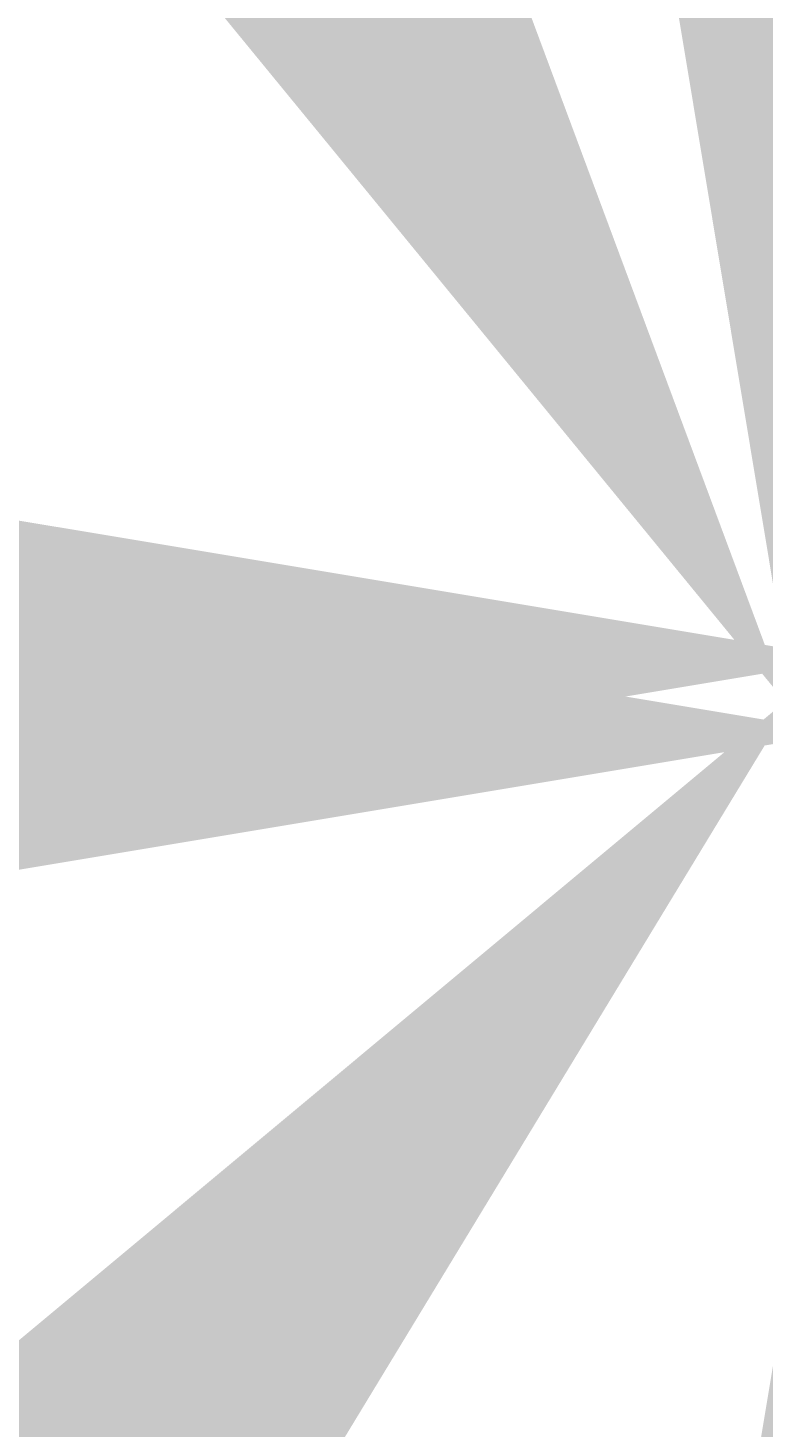
# Model space of a CAD drawing. Units: millimetres. Extents: x -22994 to 29398, y -19990 to 20176.
# Tile 4 of 135: x -2139 to -44, y -1986 to 2002. Entities that reach past the tile are written whole.
import ezdxf

# ---------------------------------------------------------------- set-up
doc = ezdxf.new("R2010")
doc.units = ezdxf.units.MM
doc.header["$MEASUREMENT"] = 0
doc.layers.add('M-DIMS', color=2, linetype='Continuous', lineweight=18)
doc.styles.get("Standard").update_dxf_attribs({"font": 'arial.ttf'})
doc.dimstyles.get("Standard").update_dxf_attribs({"dimtxt": 0.18, "dimasz": 10000, "dimexe": 0.18, "dimexo": 0.0625, "dimgap": 0.09, "dimtad": 0, "dimtih": 1, "dimtoh": 1, "dimdec": 0, "dimzin": 0, "dimdsep": 46, "dimtxsty": 'Standard', "dimcen": 0.09, "dimadec": 0, "dimazin": 0, "dimtfac": 1, "dimtdec": 0, "dimtofl": 0, "dimtmove": 0, "dimatfit": 3, "dimfxl": 1, "dimtolj": 1, "dimtzin": 0, "dimlwd": 30, "dimarcsym": 0})

# ---------------------------------------------------------------- blocks, each defined once
blk = doc.blocks.new('*D2')
at = {"layer": 'Defpoints', "color": 0, "transparency": 16777216}
for p in [(6.7, 10.3), (290.9, 10.3), (290.9, -5.1)]:
    blk.add_point(p, dxfattribs=at)
at = {"layer": 'M-DIMS', "color": 0, "lineweight": -2, "transparency": 16777216}
for p, q in [((6.7, 10.2), (6.7, -5.3)), ((290.9, 10.2), (290.9, -5.3))]:
    blk.add_line(p, q, dxfattribs=at)
at = {"layer": 'M-DIMS', "color": 0, "lineweight": 30, "transparency": 16777216}
for p, q in [((-9993.3, -5.1), (-19993.3, -5.1)), ((10290.9, -5.1), (20290.9, -5.1))]:
    blk.add_line(p, q, dxfattribs=at)
at = {"layer": 'M-DIMS', "color": 0, "transparency": 16777216}
for points in [[(-9993.3, 1661.6), (-9993.3, -1671.7), (6.7, -5.1)], [(10290.9, 1661.6), (10290.9, -1671.7), (290.9, -5.1)]]:
    blk.add_solid(points, dxfattribs=at)
at = {"layer": 'M-DIMS', "color": 0, "transparency": 16777216, "insert": (148.8, -5.1), "char_height": 0.18, "attachment_point": 5}
blk.add_mtext('\\A1;284.2', dxfattribs=at)
blk = doc.blocks.new('*D3')
at = {"layer": 'Defpoints', "color": 0, "transparency": 16777216}
for p in [(110.3, 204.2), (110.3, 176.4), (95.8, 128)]:
    blk.add_point(p, dxfattribs=at)
at = {"layer": 'M-DIMS', "color": 0, "lineweight": 30, "transparency": 16777216}
for p, q in [((-9904.2, 204.2), (-19904.2, 204.2)), ((10110.3, 204.2), (20110.3, 204.2))]:
    blk.add_line(p, q, dxfattribs=at)
at = {"layer": 'M-DIMS', "color": 0, "lineweight": -2, "transparency": 16777216}
for p, q in [((95.8, 128), (95.8, 204.3)), ((110.3, 176.4), (110.3, 204.3))]:
    blk.add_line(p, q, dxfattribs=at)
at = {"layer": 'M-DIMS', "color": 0, "transparency": 16777216}
for points in [[(-9904.2, 1870.8), (-9904.2, -1462.5), (95.8, 204.2)], [(10110.3, 1870.8), (10110.3, -1462.5), (110.3, 204.2)]]:
    blk.add_solid(points, dxfattribs=at)
at = {"layer": 'M-DIMS', "color": 0, "transparency": 16777216, "insert": (103, 204.2), "char_height": 0.18, "attachment_point": 5}
blk.add_mtext('\\A1;14.432', dxfattribs=at)
blk = doc.blocks.new('*D4')
at = {"layer": 'Defpoints', "color": 0, "transparency": 16777216}
for p in [(116.3, 204.2), (110.3, 176.4), (116.3, 176.4)]:
    blk.add_point(p, dxfattribs=at)
at = {"layer": 'M-DIMS', "color": 0, "lineweight": 30, "transparency": 16777216}
for p, q in [((-9889.7, 204.2), (-19889.7, 204.2)), ((10116.3, 204.2), (20116.3, 204.2))]:
    blk.add_line(p, q, dxfattribs=at)
at = {"layer": 'M-DIMS', "color": 0, "lineweight": -2, "transparency": 16777216}
for p, q in [((110.3, 176.4), (110.3, 204.3)), ((116.3, 176.4), (116.3, 204.3))]:
    blk.add_line(p, q, dxfattribs=at)
at = {"layer": 'M-DIMS', "color": 0, "transparency": 16777216}
for points in [[(-9889.7, 1870.8), (-9889.7, -1462.5), (110.3, 204.2)], [(10116.3, 1870.8), (10116.3, -1462.5), (116.3, 204.2)]]:
    blk.add_solid(points, dxfattribs=at)
at = {"layer": 'M-DIMS', "color": 0, "transparency": 16777216, "insert": (113.3, 204.2), "char_height": 0.18, "attachment_point": 5}
blk.add_mtext('\\A1;6', dxfattribs=at)
blk = doc.blocks.new('*D5')
at = {"layer": 'Defpoints', "color": 0, "transparency": 16777216}
for p in [(181.3, 204.2), (116.3, 176.4), (181.3, 176.4)]:
    blk.add_point(p, dxfattribs=at)
at = {"layer": 'M-DIMS', "color": 0, "lineweight": 30, "transparency": 16777216}
for p, q in [((-9883.7, 204.2), (-19883.7, 204.2)), ((10181.3, 204.2), (20181.3, 204.2))]:
    blk.add_line(p, q, dxfattribs=at)
at = {"layer": 'M-DIMS', "color": 0, "lineweight": -2, "transparency": 16777216}
for p, q in [((116.3, 176.4), (116.3, 204.3)), ((181.3, 176.4), (181.3, 204.3))]:
    blk.add_line(p, q, dxfattribs=at)
at = {"layer": 'M-DIMS', "color": 0, "transparency": 16777216}
for points in [[(-9883.7, 1870.8), (-9883.7, -1462.5), (116.3, 204.2)], [(10181.3, 1870.8), (10181.3, -1462.5), (181.3, 204.2)]]:
    blk.add_solid(points, dxfattribs=at)
at = {"layer": 'M-DIMS', "color": 0, "transparency": 16777216, "insert": (148.8, 204.2), "char_height": 0.18, "attachment_point": 5}
blk.add_mtext('\\A1;65', dxfattribs=at)
blk = doc.blocks.new('*D6')
at = {"layer": 'Defpoints', "color": 0, "transparency": 16777216}
for p in [(187.3, 204.2), (181.3, 176.4), (187.3, 176.4)]:
    blk.add_point(p, dxfattribs=at)
at = {"layer": 'M-DIMS', "color": 0, "lineweight": 30, "transparency": 16777216}
for p, q in [((-9818.7, 204.2), (-19818.7, 204.2)), ((10187.3, 204.2), (20187.3, 204.2))]:
    blk.add_line(p, q, dxfattribs=at)
at = {"layer": 'M-DIMS', "color": 0, "lineweight": -2, "transparency": 16777216}
for p, q in [((181.3, 176.4), (181.3, 204.3)), ((187.3, 176.4), (187.3, 204.3))]:
    blk.add_line(p, q, dxfattribs=at)
at = {"layer": 'M-DIMS', "color": 0, "transparency": 16777216}
for points in [[(-9818.7, 1870.8), (-9818.7, -1462.5), (181.3, 204.2)], [(10187.3, 1870.8), (10187.3, -1462.5), (187.3, 204.2)]]:
    blk.add_solid(points, dxfattribs=at)
at = {"layer": 'M-DIMS', "color": 0, "transparency": 16777216, "insert": (184.3, 204.2), "char_height": 0.18, "attachment_point": 5}
blk.add_mtext('\\A1;6', dxfattribs=at)
blk = doc.blocks.new('*D7')
at = {"layer": 'Defpoints', "color": 0, "transparency": 16777216}
for p in [(201.7, 204.2), (187.3, 176.4), (201.7, 128)]:
    blk.add_point(p, dxfattribs=at)
at = {"layer": 'M-DIMS', "color": 0, "lineweight": 30, "transparency": 16777216}
for p, q in [((-9812.7, 204.2), (-19812.7, 204.2)), ((10201.7, 204.2), (20201.7, 204.2))]:
    blk.add_line(p, q, dxfattribs=at)
at = {"layer": 'M-DIMS', "color": 0, "lineweight": -2, "transparency": 16777216}
for p, q in [((187.3, 176.4), (187.3, 204.3)), ((201.7, 128), (201.7, 204.3))]:
    blk.add_line(p, q, dxfattribs=at)
at = {"layer": 'M-DIMS', "color": 0, "transparency": 16777216}
for points in [[(-9812.7, 1870.8), (-9812.7, -1462.5), (187.3, 204.2)], [(10201.7, 1870.8), (10201.7, -1462.5), (201.7, 204.2)]]:
    blk.add_solid(points, dxfattribs=at)
at = {"layer": 'M-DIMS', "color": 0, "transparency": 16777216, "insert": (194.5, 204.2), "char_height": 0.18, "attachment_point": 5}
blk.add_mtext('\\A1;14.432', dxfattribs=at)
blk = doc.blocks.new('*D8')
at = {"layer": 'Defpoints', "color": 0, "transparency": 16777216}
for p in [(227.6, 204.2), (201.7, 128), (227.6, 146.7)]:
    blk.add_point(p, dxfattribs=at)
at = {"layer": 'M-DIMS', "color": 0, "lineweight": 30, "transparency": 16777216}
for p, q in [((-9798.3, 204.2), (-19798.3, 204.2)), ((10227.6, 204.2), (20227.6, 204.2))]:
    blk.add_line(p, q, dxfattribs=at)
at = {"layer": 'M-DIMS', "color": 0, "lineweight": -2, "transparency": 16777216}
for p, q in [((201.7, 128), (201.7, 204.3)), ((227.6, 146.8), (227.6, 204.3))]:
    blk.add_line(p, q, dxfattribs=at)
at = {"layer": 'M-DIMS', "color": 0, "transparency": 16777216}
for points in [[(-9798.3, 1870.8), (-9798.3, -1462.5), (201.7, 204.2)], [(10227.6, 1870.8), (10227.6, -1462.5), (227.6, 204.2)]]:
    blk.add_solid(points, dxfattribs=at)
at = {"layer": 'M-DIMS', "color": 0, "transparency": 16777216, "insert": (214.7, 204.2), "char_height": 0.18, "attachment_point": 5}
blk.add_mtext('\\A1;25.95', dxfattribs=at)
blk = doc.blocks.new('*D9')
at = {"layer": 'Defpoints', "color": 0, "transparency": 16777216}
for p in [(187.3, 176.4), (306.2, 176.4), (290.9, 10.3)]:
    blk.add_point(p, dxfattribs=at)
at = {"layer": 'M-DIMS', "color": 0, "lineweight": 30, "transparency": 16777216}
for p, q in [((306.2, 10176.4), (306.2, 20176.4)), ((306.2, -9989.7), (306.2, -19989.7))]:
    blk.add_line(p, q, dxfattribs=at)
at = {"layer": 'M-DIMS', "color": 0, "lineweight": -2, "transparency": 16777216}
for p, q in [((187.3, 176.4), (306.4, 176.4)), ((290.9, 10.3), (306.4, 10.3))]:
    blk.add_line(p, q, dxfattribs=at)
at = {"layer": 'M-DIMS', "color": 0, "transparency": 16777216}
for points in [[(-1360.5, 10176.4), (1972.9, 10176.4), (306.2, 176.4)], [(-1360.5, -9989.7), (1972.9, -9989.7), (306.2, 10.3)]]:
    blk.add_solid(points, dxfattribs=at)
at = {"layer": 'M-DIMS', "color": 0, "transparency": 16777216, "insert": (306.2, 93.3), "char_height": 0.18, "attachment_point": 5}
blk.add_mtext('\\A1;166.1', dxfattribs=at)
blk = doc.blocks.new('*D10')
at = {"layer": 'Defpoints', "color": 0, "transparency": 16777216}
for p in [(125.6, 136.1), (133.3, 136.1), (133.3, -5.1)]:
    blk.add_point(p, dxfattribs=at)
at = {"layer": 'M-DIMS', "color": 0, "lineweight": -2, "transparency": 16777216}
for p, q in [((125.6, 136), (125.6, -5.3)), ((133.3, 136), (133.3, -5.3))]:
    blk.add_line(p, q, dxfattribs=at)
at = {"layer": 'M-DIMS', "color": 0, "lineweight": 30, "transparency": 16777216}
for p, q in [((-9874.4, -5.1), (-19874.4, -5.1)), ((10133.3, -5.1), (20133.3, -5.1))]:
    blk.add_line(p, q, dxfattribs=at)
at = {"layer": 'M-DIMS', "color": 0, "transparency": 16777216}
for points in [[(-9874.4, 1661.6), (-9874.4, -1671.7), (125.6, -5.1)], [(10133.3, 1661.6), (10133.3, -1671.7), (133.3, -5.1)]]:
    blk.add_solid(points, dxfattribs=at)
at = {"layer": 'M-DIMS', "color": 0, "transparency": 16777216, "insert": (129.5, -5.1), "char_height": 0.18, "attachment_point": 5}
blk.add_mtext('\\A1;7.696', dxfattribs=at)
blk = doc.blocks.new('*D11')
at = {"layer": 'Defpoints', "color": 0, "transparency": 16777216}
for p in [(133.3, 136.1), (135.6, 136.1), (135.6, -5.1)]:
    blk.add_point(p, dxfattribs=at)
at = {"layer": 'M-DIMS', "color": 0, "lineweight": -2, "transparency": 16777216}
for p, q in [((133.3, 136), (133.3, -5.3)), ((135.6, 136), (135.6, -5.3))]:
    blk.add_line(p, q, dxfattribs=at)
at = {"layer": 'M-DIMS', "color": 0, "lineweight": 30, "transparency": 16777216}
for p, q in [((-9866.7, -5.1), (-19866.7, -5.1)), ((10135.6, -5.1), (20135.6, -5.1))]:
    blk.add_line(p, q, dxfattribs=at)
at = {"layer": 'M-DIMS', "color": 0, "transparency": 16777216}
for points in [[(-9866.7, 1661.6), (-9866.7, -1671.7), (133.3, -5.1)], [(10135.6, 1661.6), (10135.6, -1671.7), (135.6, -5.1)]]:
    blk.add_solid(points, dxfattribs=at)
at = {"layer": 'M-DIMS', "color": 0, "transparency": 16777216, "insert": (134.5, -5.1), "char_height": 0.18, "attachment_point": 5}
blk.add_mtext('\\A1;2.304', dxfattribs=at)
blk = doc.blocks.new('*D12')
at = {"layer": 'Defpoints', "color": 0, "transparency": 16777216}
for p in [(135.6, 136.1), (145.6, 136.1), (145.6, -5.1)]:
    blk.add_point(p, dxfattribs=at)
at = {"layer": 'M-DIMS', "color": 0, "lineweight": -2, "transparency": 16777216}
for p, q in [((135.6, 136), (135.6, -5.3)), ((145.6, 136), (145.6, -5.3))]:
    blk.add_line(p, q, dxfattribs=at)
at = {"layer": 'M-DIMS', "color": 0, "lineweight": 30, "transparency": 16777216}
for p, q in [((-9864.4, -5.1), (-19864.4, -5.1)), ((10145.6, -5.1), (20145.6, -5.1))]:
    blk.add_line(p, q, dxfattribs=at)
at = {"layer": 'M-DIMS', "color": 0, "transparency": 16777216}
for points in [[(-9864.4, 1661.6), (-9864.4, -1671.7), (135.6, -5.1)], [(10145.6, 1661.6), (10145.6, -1671.7), (145.6, -5.1)]]:
    blk.add_solid(points, dxfattribs=at)
at = {"layer": 'M-DIMS', "color": 0, "transparency": 16777216, "insert": (140.6, -5.1), "char_height": 0.18, "attachment_point": 5}
blk.add_mtext('\\A1;10', dxfattribs=at)
blk = doc.blocks.new('*D13')
at = {"layer": 'Defpoints', "color": 0, "transparency": 16777216}
for p in [(145.6, 136.1), (155.6, 136.1), (155.6, -5.1)]:
    blk.add_point(p, dxfattribs=at)
at = {"layer": 'M-DIMS', "color": 0, "lineweight": -2, "transparency": 16777216}
for p, q in [((145.6, 136), (145.6, -5.3)), ((155.6, 136), (155.6, -5.3))]:
    blk.add_line(p, q, dxfattribs=at)
at = {"layer": 'M-DIMS', "color": 0, "lineweight": 30, "transparency": 16777216}
for p, q in [((-9854.4, -5.1), (-19854.4, -5.1)), ((10155.6, -5.1), (20155.6, -5.1))]:
    blk.add_line(p, q, dxfattribs=at)
at = {"layer": 'M-DIMS', "color": 0, "transparency": 16777216}
for points in [[(-9854.4, 1661.6), (-9854.4, -1671.7), (145.6, -5.1)], [(10155.6, 1661.6), (10155.6, -1671.7), (155.6, -5.1)]]:
    blk.add_solid(points, dxfattribs=at)
at = {"layer": 'M-DIMS', "color": 0, "transparency": 16777216, "insert": (150.6, -5.1), "char_height": 0.18, "attachment_point": 5}
blk.add_mtext('\\A1;10', dxfattribs=at)
blk = doc.blocks.new('*D14')
at = {"layer": 'Defpoints', "color": 0, "transparency": 16777216}
for p in [(155.6, 136.1), (165.6, 136.1), (165.6, -5.1)]:
    blk.add_point(p, dxfattribs=at)
at = {"layer": 'M-DIMS', "color": 0, "lineweight": -2, "transparency": 16777216}
for p, q in [((155.6, 136), (155.6, -5.3)), ((165.6, 136), (165.6, -5.3))]:
    blk.add_line(p, q, dxfattribs=at)
at = {"layer": 'M-DIMS', "color": 0, "lineweight": 30, "transparency": 16777216}
for p, q in [((-9844.4, -5.1), (-19844.4, -5.1)), ((10165.6, -5.1), (20165.6, -5.1))]:
    blk.add_line(p, q, dxfattribs=at)
at = {"layer": 'M-DIMS', "color": 0, "transparency": 16777216}
for points in [[(-9844.4, 1661.6), (-9844.4, -1671.7), (155.6, -5.1)], [(10165.6, 1661.6), (10165.6, -1671.7), (165.6, -5.1)]]:
    blk.add_solid(points, dxfattribs=at)
at = {"layer": 'M-DIMS', "color": 0, "transparency": 16777216, "insert": (160.6, -5.1), "char_height": 0.18, "attachment_point": 5}
blk.add_mtext('\\A1;10', dxfattribs=at)
blk = doc.blocks.new('*D15')
at = {"layer": 'Defpoints', "color": 0, "transparency": 16777216}
for p in [(173.3, 154.8), (173.3, 136.1), (306.2, 136.1)]:
    blk.add_point(p, dxfattribs=at)
at = {"layer": 'M-DIMS', "color": 0, "lineweight": 30, "transparency": 16777216}
for p, q in [((306.2, 10154.8), (306.2, 20154.8)), ((306.2, -9863.9), (306.2, -19863.9))]:
    blk.add_line(p, q, dxfattribs=at)
at = {"layer": 'M-DIMS', "color": 0, "lineweight": -2, "transparency": 16777216}
for p, q in [((173.4, 154.8), (306.4, 154.8)), ((173.4, 136.1), (306.4, 136.1))]:
    blk.add_line(p, q, dxfattribs=at)
at = {"layer": 'M-DIMS', "color": 0, "transparency": 16777216}
for points in [[(-1360.5, 10154.8), (1972.9, 10154.8), (306.2, 154.8)], [(-1360.5, -9863.9), (1972.9, -9863.9), (306.2, 136.1)]]:
    blk.add_solid(points, dxfattribs=at)
at = {"layer": 'M-DIMS', "color": 0, "transparency": 16777216, "insert": (306.2, 145.4), "char_height": 0.18, "attachment_point": 5}
blk.add_mtext('\\A1;18.717', dxfattribs=at)
blk = doc.blocks.new('*D16')
at = {"layer": 'Defpoints', "color": 0, "transparency": 16777216}
for p in [(120.2, 204.2), (110.5, 48), (120.2, 48)]:
    blk.add_point(p, dxfattribs=at)
at = {"layer": 'M-DIMS', "color": 0, "lineweight": 30, "transparency": 16777216}
for p, q in [((-9889.5, 204.2), (-19889.5, 204.2)), ((10120.2, 204.2), (20120.2, 204.2))]:
    blk.add_line(p, q, dxfattribs=at)
at = {"layer": 'M-DIMS', "color": 0, "lineweight": -2, "transparency": 16777216}
for p, q in [((110.5, 48.1), (110.5, 204.3)), ((120.2, 48.1), (120.2, 204.3))]:
    blk.add_line(p, q, dxfattribs=at)
at = {"layer": 'M-DIMS', "color": 0, "transparency": 16777216}
for points in [[(-9889.5, 1870.8), (-9889.5, -1462.5), (110.5, 204.2)], [(10120.2, 1870.8), (10120.2, -1462.5), (120.2, 204.2)]]:
    blk.add_solid(points, dxfattribs=at)
at = {"layer": 'M-DIMS', "color": 0, "transparency": 16777216, "insert": (115.3, 204.2), "char_height": 0.18, "attachment_point": 5}
blk.add_mtext('\\A1;9.704', dxfattribs=at)
blk = doc.blocks.new('*D17')
at = {"layer": 'Defpoints', "color": 0, "transparency": 16777216}
for p in [(126.2, 204.2), (120.2, 48), (126.2, 48)]:
    blk.add_point(p, dxfattribs=at)
at = {"layer": 'M-DIMS', "color": 0, "lineweight": 30, "transparency": 16777216}
for p, q in [((-9879.8, 204.2), (-19879.8, 204.2)), ((10126.2, 204.2), (20126.2, 204.2))]:
    blk.add_line(p, q, dxfattribs=at)
at = {"layer": 'M-DIMS', "color": 0, "lineweight": -2, "transparency": 16777216}
for p, q in [((120.2, 48.1), (120.2, 204.3)), ((126.2, 48.1), (126.2, 204.3))]:
    blk.add_line(p, q, dxfattribs=at)
at = {"layer": 'M-DIMS', "color": 0, "transparency": 16777216}
for points in [[(-9879.8, 1870.8), (-9879.8, -1462.5), (120.2, 204.2)], [(10126.2, 1870.8), (10126.2, -1462.5), (126.2, 204.2)]]:
    blk.add_solid(points, dxfattribs=at)
at = {"layer": 'M-DIMS', "color": 0, "transparency": 16777216, "insert": (123.2, 204.2), "char_height": 0.18, "attachment_point": 5}
blk.add_mtext('\\A1;6', dxfattribs=at)
blk = doc.blocks.new('*D18')
at = {"layer": 'Defpoints', "color": 0, "transparency": 16777216}
for p in [(132.2, 204.2), (126.2, 48), (132.2, 48)]:
    blk.add_point(p, dxfattribs=at)
at = {"layer": 'M-DIMS', "color": 0, "lineweight": 30, "transparency": 16777216}
for p, q in [((-9873.8, 204.2), (-19873.8, 204.2)), ((10132.2, 204.2), (20132.2, 204.2))]:
    blk.add_line(p, q, dxfattribs=at)
at = {"layer": 'M-DIMS', "color": 0, "lineweight": -2, "transparency": 16777216}
for p, q in [((126.2, 48.1), (126.2, 204.3)), ((132.2, 48.1), (132.2, 204.3))]:
    blk.add_line(p, q, dxfattribs=at)
at = {"layer": 'M-DIMS', "color": 0, "transparency": 16777216}
for points in [[(-9873.8, 1870.8), (-9873.8, -1462.5), (126.2, 204.2)], [(10132.2, 1870.8), (10132.2, -1462.5), (132.2, 204.2)]]:
    blk.add_solid(points, dxfattribs=at)
at = {"layer": 'M-DIMS', "color": 0, "transparency": 16777216, "insert": (129.2, 204.2), "char_height": 0.18, "attachment_point": 5}
blk.add_mtext('\\A1;6', dxfattribs=at)
blk = doc.blocks.new('*D19')
at = {"layer": 'Defpoints', "color": 0, "transparency": 16777216}
for p in [(138.2, 204.2), (132.2, 48), (138.2, 48)]:
    blk.add_point(p, dxfattribs=at)
at = {"layer": 'M-DIMS', "color": 0, "lineweight": 30, "transparency": 16777216}
for p, q in [((-9867.8, 204.2), (-19867.8, 204.2)), ((10138.2, 204.2), (20138.2, 204.2))]:
    blk.add_line(p, q, dxfattribs=at)
at = {"layer": 'M-DIMS', "color": 0, "lineweight": -2, "transparency": 16777216}
for p, q in [((132.2, 48.1), (132.2, 204.3)), ((138.2, 48.1), (138.2, 204.3))]:
    blk.add_line(p, q, dxfattribs=at)
at = {"layer": 'M-DIMS', "color": 0, "transparency": 16777216}
for points in [[(-9867.8, 1870.8), (-9867.8, -1462.5), (132.2, 204.2)], [(10138.2, 1870.8), (10138.2, -1462.5), (138.2, 204.2)]]:
    blk.add_solid(points, dxfattribs=at)
at = {"layer": 'M-DIMS', "color": 0, "transparency": 16777216, "insert": (135.2, 204.2), "char_height": 0.18, "attachment_point": 5}
blk.add_mtext('\\A1;6', dxfattribs=at)
blk = doc.blocks.new('*D20')
at = {"layer": 'Defpoints', "color": 0, "transparency": 16777216}
for p in [(144.2, 204.2), (138.2, 48), (144.2, 48)]:
    blk.add_point(p, dxfattribs=at)
at = {"layer": 'M-DIMS', "color": 0, "lineweight": 30, "transparency": 16777216}
for p, q in [((-9861.8, 204.2), (-19861.8, 204.2)), ((10144.2, 204.2), (20144.2, 204.2))]:
    blk.add_line(p, q, dxfattribs=at)
at = {"layer": 'M-DIMS', "color": 0, "lineweight": -2, "transparency": 16777216}
for p, q in [((138.2, 48.1), (138.2, 204.3)), ((144.2, 48.1), (144.2, 204.3))]:
    blk.add_line(p, q, dxfattribs=at)
at = {"layer": 'M-DIMS', "color": 0, "transparency": 16777216}
for points in [[(-9861.8, 1870.8), (-9861.8, -1462.5), (138.2, 204.2)], [(10144.2, 1870.8), (10144.2, -1462.5), (144.2, 204.2)]]:
    blk.add_solid(points, dxfattribs=at)
at = {"layer": 'M-DIMS', "color": 0, "transparency": 16777216, "insert": (141.2, 204.2), "char_height": 0.18, "attachment_point": 5}
blk.add_mtext('\\A1;6', dxfattribs=at)
blk = doc.blocks.new('*D21')
at = {"layer": 'Defpoints', "color": 0, "transparency": 16777216}
for p in [(149.1, 204.2), (144.2, 48), (149.1, 48)]:
    blk.add_point(p, dxfattribs=at)
at = {"layer": 'M-DIMS', "color": 0, "lineweight": 30, "transparency": 16777216}
for p, q in [((-9855.8, 204.2), (-19855.8, 204.2)), ((10149.1, 204.2), (20149.1, 204.2))]:
    blk.add_line(p, q, dxfattribs=at)
at = {"layer": 'M-DIMS', "color": 0, "lineweight": -2, "transparency": 16777216}
for p, q in [((144.2, 48.1), (144.2, 204.3)), ((149.1, 48.1), (149.1, 204.3))]:
    blk.add_line(p, q, dxfattribs=at)
at = {"layer": 'M-DIMS', "color": 0, "transparency": 16777216}
for points in [[(-9855.8, 1870.8), (-9855.8, -1462.5), (144.2, 204.2)], [(10149.1, 1870.8), (10149.1, -1462.5), (149.1, 204.2)]]:
    blk.add_solid(points, dxfattribs=at)
at = {"layer": 'M-DIMS', "color": 0, "transparency": 16777216, "insert": (146.6, 204.2), "char_height": 0.18, "attachment_point": 5}
blk.add_mtext('\\A1;4.945', dxfattribs=at)
blk = doc.blocks.new('*D22')
at = {"layer": 'Defpoints', "color": 0, "transparency": 16777216}
for p in [(149.1, 31), (155.1, 31), (155.1, -5.1)]:
    blk.add_point(p, dxfattribs=at)
at = {"layer": 'M-DIMS', "color": 0, "lineweight": -2, "transparency": 16777216}
for p, q in [((149.1, 30.9), (149.1, -5.3)), ((155.1, 30.9), (155.1, -5.3))]:
    blk.add_line(p, q, dxfattribs=at)
at = {"layer": 'M-DIMS', "color": 0, "lineweight": 30, "transparency": 16777216}
for p, q in [((-9850.9, -5.1), (-19850.9, -5.1)), ((10155.1, -5.1), (20155.1, -5.1))]:
    blk.add_line(p, q, dxfattribs=at)
at = {"layer": 'M-DIMS', "color": 0, "transparency": 16777216}
for points in [[(-9850.9, 1661.6), (-9850.9, -1671.7), (149.1, -5.1)], [(10155.1, 1661.6), (10155.1, -1671.7), (155.1, -5.1)]]:
    blk.add_solid(points, dxfattribs=at)
at = {"layer": 'M-DIMS', "color": 0, "transparency": 16777216, "insert": (152.1, -5.1), "char_height": 0.18, "attachment_point": 5}
blk.add_mtext('\\A1;6', dxfattribs=at)
blk = doc.blocks.new('*D23')
at = {"layer": 'Defpoints', "color": 0, "transparency": 16777216}
for p in [(155.1, 31), (161.1, 31), (161.1, -5.1)]:
    blk.add_point(p, dxfattribs=at)
at = {"layer": 'M-DIMS', "color": 0, "lineweight": -2, "transparency": 16777216}
for p, q in [((155.1, 30.9), (155.1, -5.3)), ((161.1, 30.9), (161.1, -5.3))]:
    blk.add_line(p, q, dxfattribs=at)
at = {"layer": 'M-DIMS', "color": 0, "lineweight": 30, "transparency": 16777216}
for p, q in [((-9844.9, -5.1), (-19844.9, -5.1)), ((10161.1, -5.1), (20161.1, -5.1))]:
    blk.add_line(p, q, dxfattribs=at)
at = {"layer": 'M-DIMS', "color": 0, "transparency": 16777216}
for points in [[(-9844.9, 1661.6), (-9844.9, -1671.7), (155.1, -5.1)], [(10161.1, 1661.6), (10161.1, -1671.7), (161.1, -5.1)]]:
    blk.add_solid(points, dxfattribs=at)
at = {"layer": 'M-DIMS', "color": 0, "transparency": 16777216, "insert": (158.1, -5.1), "char_height": 0.18, "attachment_point": 5}
blk.add_mtext('\\A1;6', dxfattribs=at)
blk = doc.blocks.new('*D24')
at = {"layer": 'Defpoints', "color": 0, "transparency": 16777216}
for p in [(161.1, 31), (166.4, 31), (166.4, -5.1)]:
    blk.add_point(p, dxfattribs=at)
at = {"layer": 'M-DIMS', "color": 0, "lineweight": -2, "transparency": 16777216}
for p, q in [((161.1, 30.9), (161.1, -5.3)), ((166.4, 30.9), (166.4, -5.3))]:
    blk.add_line(p, q, dxfattribs=at)
at = {"layer": 'M-DIMS', "color": 0, "lineweight": 30, "transparency": 16777216}
for p, q in [((-9838.9, -5.1), (-19838.9, -5.1)), ((10166.4, -5.1), (20166.4, -5.1))]:
    blk.add_line(p, q, dxfattribs=at)
at = {"layer": 'M-DIMS', "color": 0, "transparency": 16777216}
for points in [[(-9838.9, 1661.6), (-9838.9, -1671.7), (161.1, -5.1)], [(10166.4, 1661.6), (10166.4, -1671.7), (166.4, -5.1)]]:
    blk.add_solid(points, dxfattribs=at)
at = {"layer": 'M-DIMS', "color": 0, "transparency": 16777216, "insert": (163.8, -5.1), "char_height": 0.18, "attachment_point": 5}
blk.add_mtext('\\A1;5.323', dxfattribs=at)
blk = doc.blocks.new('*D25')
at = {"layer": 'Defpoints', "color": 0, "transparency": 16777216}
for p in [(166.4, 31), (172.4, 31), (172.4, -5.1)]:
    blk.add_point(p, dxfattribs=at)
at = {"layer": 'M-DIMS', "color": 0, "lineweight": -2, "transparency": 16777216}
for p, q in [((166.4, 30.9), (166.4, -5.3)), ((172.4, 30.9), (172.4, -5.3))]:
    blk.add_line(p, q, dxfattribs=at)
at = {"layer": 'M-DIMS', "color": 0, "lineweight": 30, "transparency": 16777216}
for p, q in [((-9833.6, -5.1), (-19833.6, -5.1)), ((10172.4, -5.1), (20172.4, -5.1))]:
    blk.add_line(p, q, dxfattribs=at)
at = {"layer": 'M-DIMS', "color": 0, "transparency": 16777216}
for points in [[(-9833.6, 1661.6), (-9833.6, -1671.7), (166.4, -5.1)], [(10172.4, 1661.6), (10172.4, -1671.7), (172.4, -5.1)]]:
    blk.add_solid(points, dxfattribs=at)
at = {"layer": 'M-DIMS', "color": 0, "transparency": 16777216, "insert": (169.4, -5.1), "char_height": 0.18, "attachment_point": 5}
blk.add_mtext('\\A1;6', dxfattribs=at)
blk = doc.blocks.new('*D26')
at = {"layer": 'Defpoints', "color": 0, "transparency": 16777216}
for p in [(172.4, 31), (178.4, 31), (178.4, -5.1)]:
    blk.add_point(p, dxfattribs=at)
at = {"layer": 'M-DIMS', "color": 0, "lineweight": -2, "transparency": 16777216}
for p, q in [((172.4, 30.9), (172.4, -5.3)), ((178.4, 30.9), (178.4, -5.3))]:
    blk.add_line(p, q, dxfattribs=at)
at = {"layer": 'M-DIMS', "color": 0, "lineweight": 30, "transparency": 16777216}
for p, q in [((-9827.6, -5.1), (-19827.6, -5.1)), ((10178.4, -5.1), (20178.4, -5.1))]:
    blk.add_line(p, q, dxfattribs=at)
at = {"layer": 'M-DIMS', "color": 0, "transparency": 16777216}
for points in [[(-9827.6, 1661.6), (-9827.6, -1671.7), (172.4, -5.1)], [(10178.4, 1661.6), (10178.4, -1671.7), (178.4, -5.1)]]:
    blk.add_solid(points, dxfattribs=at)
at = {"layer": 'M-DIMS', "color": 0, "transparency": 16777216, "insert": (175.4, -5.1), "char_height": 0.18, "attachment_point": 5}
blk.add_mtext('\\A1;6', dxfattribs=at)
blk = doc.blocks.new('*D27')
at = {"layer": 'Defpoints', "color": 0, "transparency": 16777216}
for p in [(178.4, 31), (188.1, 31), (188.1, -5.1)]:
    blk.add_point(p, dxfattribs=at)
at = {"layer": 'M-DIMS', "color": 0, "lineweight": -2, "transparency": 16777216}
for p, q in [((178.4, 30.9), (178.4, -5.3)), ((188.1, 30.9), (188.1, -5.3))]:
    blk.add_line(p, q, dxfattribs=at)
at = {"layer": 'M-DIMS', "color": 0, "lineweight": 30, "transparency": 16777216}
for p, q in [((-9821.6, -5.1), (-19821.6, -5.1)), ((10188.1, -5.1), (20188.1, -5.1))]:
    blk.add_line(p, q, dxfattribs=at)
at = {"layer": 'M-DIMS', "color": 0, "transparency": 16777216}
for points in [[(-9821.6, 1661.6), (-9821.6, -1671.7), (178.4, -5.1)], [(10188.1, 1661.6), (10188.1, -1671.7), (188.1, -5.1)]]:
    blk.add_solid(points, dxfattribs=at)
at = {"layer": 'M-DIMS', "color": 0, "transparency": 16777216, "insert": (183.3, -5.1), "char_height": 0.18, "attachment_point": 5}
blk.add_mtext('\\A1;9.679', dxfattribs=at)
blk = doc.blocks.new('*D28')
at = {"layer": 'Defpoints', "color": 0, "transparency": 16777216}
for p in [(188.1, 48), (306.2, 48), (188.1, 31)]:
    blk.add_point(p, dxfattribs=at)
at = {"layer": 'M-DIMS', "color": 0, "lineweight": 30, "transparency": 16777216}
for p, q in [((306.2, 10048), (306.2, 20048)), ((306.2, -9969), (306.2, -19969))]:
    blk.add_line(p, q, dxfattribs=at)
at = {"layer": 'M-DIMS', "color": 0, "lineweight": -2, "transparency": 16777216}
for p, q in [((188.2, 48), (306.4, 48)), ((188.2, 31), (306.4, 31))]:
    blk.add_line(p, q, dxfattribs=at)
at = {"layer": 'M-DIMS', "color": 0, "transparency": 16777216}
for points in [[(-1360.5, 10048), (1972.9, 10048), (306.2, 48)], [(-1360.5, -9969), (1972.9, -9969), (306.2, 31)]]:
    blk.add_solid(points, dxfattribs=at)
at = {"layer": 'M-DIMS', "color": 0, "transparency": 16777216, "insert": (306.2, 39.5), "char_height": 0.18, "attachment_point": 5}
blk.add_mtext('\\A1;17.045', dxfattribs=at)
blk = doc.blocks.new('*D32')
at = {"layer": 'Defpoints', "color": 0, "transparency": 16777216}
for p in [(52.4, 113.1), (57.2, 118.6)]:
    blk.add_point(p, dxfattribs=at)
at = {"layer": 'M-DIMS', "color": 0, "lineweight": -2, "transparency": 16777216}
for p, q in [((57.1, 118.6), (57.3, 118.6)), ((57.2, 118.5), (57.2, 118.7))]:
    blk.add_line(p, q, dxfattribs=at)
at = {"layer": 'M-DIMS', "color": 0, "lineweight": 30, "transparency": 16777216}
for p, q in [((-12992.5, -15047), (-6470.1, -7467)), ((-22992.5, -15047), (-12992.5, -15047))]:
    blk.add_line(p, q, dxfattribs=at)
at = {"layer": 'M-DIMS', "color": 0, "transparency": 16777216}
blk.add_solid([(-7733.4, -6379.9), (-5206.7, -8554), (52.4, 113.1)], dxfattribs=at)
at = {"layer": 'M-DIMS', "color": 0, "transparency": 16777216, "insert": (-22993.2, -15047), "char_height": 0.18, "attachment_point": 5}
blk.add_mtext('\\A1;2X R7.284', dxfattribs=at)
blk = doc.blocks.new('*D35')
at = {"layer": 'Defpoints', "color": 0, "transparency": 16777216}
for p in [(21.1, 77.4), (21.8, 76.1)]:
    blk.add_point(p, dxfattribs=at)
at = {"layer": 'M-DIMS', "color": 0, "lineweight": 30, "transparency": 16777216}
for p, q in [((-19938, 17421.4), (-9938, 17421.4)), ((-9938, 17421.4), (-4958.5, 8749.4))]:
    blk.add_line(p, q, dxfattribs=at)
at = {"layer": 'M-DIMS', "color": 0, "lineweight": -2, "transparency": 16777216}
for p, q in [((21.8, 76), (21.8, 76.2)), ((21.8, 76.1), (21.9, 76.1))]:
    blk.add_line(p, q, dxfattribs=at)
at = {"layer": 'M-DIMS', "color": 0, "transparency": 16777216}
blk.add_solid([(-3513.1, 9579.3), (-6403.8, 7919.5), (21.1, 77.4)], dxfattribs=at)
at = {"layer": 'M-DIMS', "color": 0, "transparency": 16777216, "insert": (-19938.4, 17421.4), "char_height": 0.18, "attachment_point": 5}
blk.add_mtext('\\A1;R1.5', dxfattribs=at)
blk = doc.blocks.new('*D36')
at = {"layer": 'Defpoints', "color": 0, "transparency": 16777216}
for p in [(46.4, 31.3), (46.4, 26.6)]:
    blk.add_point(p, dxfattribs=at)
at = {"layer": 'M-DIMS', "color": 0, "lineweight": 30, "transparency": 16777216}
for p, q in [((57.1, 20031.3), (51.8, 10031.3)), ((10057.1, 20031.3), (57.1, 20031.3))]:
    blk.add_line(p, q, dxfattribs=at)
at = {"layer": 'M-DIMS', "color": 0, "lineweight": -2, "transparency": 16777216}
for p, q in [((46.3, 28.9), (46.5, 28.9)), ((46.4, 28.9), (46.4, 29))]:
    blk.add_line(p, q, dxfattribs=at)
at = {"layer": 'M-DIMS', "color": 0, "transparency": 16777216}
blk.add_solid([(-1614.9, 10032.2), (1718.4, 10030.4), (46.4, 31.3)], dxfattribs=at)
at = {"layer": 'M-DIMS', "color": 0, "transparency": 16777216, "insert": (10057.6, 20031.3), "char_height": 0.18, "attachment_point": 5}
blk.add_mtext('\\A1;∅4.71', dxfattribs=at)

msp = doc.modelspace()

# ---------------------------------------------------------------- dimensions: what is measured, and where the dimension line sits
at = {"layer": 'M-DIMS'}
for base, p1, p2, override, picture, middle in [((306.202, 176.3662), (290.852, 10.2713), (187.2647, 176.3662), {"dimdec": 1, "dimlfac": 1, "dimrnd": 0, "dimzin": 0, "dimdsep": 46, "dimlunit": 2}, '*D9', (306.202, 93.3187)), ((306.202, 136.0713), (173.3459, 154.788), (173.3459, 136.0713), {"dimdec": 3, "dimlfac": 1, "dimrnd": 0, "dimzin": 0, "dimdsep": 46, "dimlunit": 2}, '*D15', (306.202, 145.4297)), ((306.202, 48.0349), (188.1175, 30.9895), (188.1175, 48.0349), {"dimdec": 3, "dimlfac": 1, "dimrnd": 0, "dimzin": 0, "dimdsep": 46, "dimlunit": 2}, '*D28', (306.202, 39.5122))]:
    dim = msp.add_linear_dim(base=base, p1=p1, p2=p2, angle=90, dimstyle='Standard', override=override, dxfattribs=at)
    dim.commit()
    dim.dimension.update_dxf_attribs({"geometry": picture, "text_midpoint": middle})
dim = msp.add_diameter_dim_2p(p1=(46.3875, 26.5934), p2=(46.39, 31.3035), dimstyle='Standard', override={"dimdec": 2, "dimlfac": 1, "dimrnd": 0, "dimzin": 0, "dimdsep": 46, "dimlunit": 2}, dxfattribs=at)
dim.commit()
dim.dimension.update_dxf_attribs({"geometry": '*D36', "text_midpoint": (10057.5542, 20031.3006), "dimtype": 163})
dim = msp.add_radius_dim(center=(21.8402, 76.0922), mpoint=(21.0933, 77.393), dimstyle='Standard', override={"dimdec": 1, "dimlfac": 1, "dimrnd": 0, "dimzin": 0, "dimdsep": 46, "dimlunit": 2}, dxfattribs=at)
dim.commit()
dim.dimension.update_dxf_attribs({"geometry": '*D35', "text_midpoint": (-19938.3541, 17421.4466)})
for base, p1, p2, override, picture, middle in [((110.2647, 204.1654), (95.8327, 127.967), (110.2647, 176.3662), {"dimdec": 3, "dimlfac": 1, "dimrnd": 0, "dimzin": 0, "dimdsep": 46, "dimlunit": 2}, '*D3', (103.0487, 204.1654)), ((116.2647, 204.1654), (110.2647, 176.3662), (116.2647, 176.3662), {"dimdec": 0, "dimlfac": 1, "dimrnd": 0, "dimzin": 0, "dimdsep": 46, "dimlunit": 2}, '*D4', (113.2647, 204.1654)), ((120.1702, 204.1654), (110.4658, 48.0349), (120.1702, 48.0349), {"dimdec": 3, "dimlfac": 1, "dimrnd": 0, "dimzin": 0, "dimdsep": 46, "dimlunit": 2}, '*D16', (115.318, 204.1654)), ((181.2647, 204.1654), (116.2647, 176.3662), (181.2647, 176.3662), {"dimdec": 0, "dimlfac": 1, "dimrnd": 0, "dimzin": 0, "dimdsep": 46, "dimlunit": 2}, '*D5', (148.7647, 204.1654)), ((126.1702, 204.1654), (120.1702, 48.0349), (126.1702, 48.0349), {"dimdec": 0, "dimlfac": 1, "dimrnd": 0, "dimzin": 0, "dimdsep": 46, "dimlunit": 2}, '*D17', (123.1702, 204.1654)), ((132.1702, 204.1654), (126.1702, 48.0349), (132.1702, 48.0349), {"dimdec": 0, "dimlfac": 1, "dimrnd": 0, "dimzin": 0, "dimdsep": 46, "dimlunit": 2}, '*D18', (129.1702, 204.1654)), ((138.1702, 204.1654), (132.1702, 48.0349), (138.1702, 48.0349), {"dimdec": 0, "dimlfac": 1, "dimrnd": 0, "dimzin": 0, "dimdsep": 46, "dimlunit": 2}, '*D19', (135.1702, 204.1654)), ((144.1702, 204.1654), (138.1702, 48.0349), (144.1702, 48.0349), {"dimdec": 0, "dimlfac": 1, "dimrnd": 0, "dimzin": 0, "dimdsep": 46, "dimlunit": 2}, '*D20', (141.1702, 204.1654)), ((149.11567, 204.16539), (144.17023, 48.03494), (149.11567, 48.03494), {"dimdec": 3, "dimlfac": 1, "dimrnd": 0, "dimzin": 0, "dimdsep": 46, "dimlunit": 2}, '*D21', (146.64295, 204.16539)), ((187.2647, 204.1654), (181.2647, 176.3662), (187.2647, 176.3662), {"dimdec": 0, "dimlfac": 1, "dimrnd": 0, "dimzin": 0, "dimdsep": 46, "dimlunit": 2}, '*D6', (184.2647, 204.1654)), ((201.6967, 204.1654), (187.2647, 176.3662), (201.6967, 127.967), {"dimdec": 3, "dimlfac": 1, "dimrnd": 0, "dimzin": 0, "dimdsep": 46, "dimlunit": 2}, '*D7', (194.4807, 204.1654)), ((227.6485, 204.1654), (201.6967, 127.967), (227.6485, 146.7296), {"dimdec": 2, "dimlfac": 1, "dimrnd": 0, "dimzin": 0, "dimdsep": 46, "dimlunit": 2}, '*D8', (214.6726, 204.1654)), ((290.852, -5.0787), (6.6773, 10.2713), (290.852, 10.2713), {"dimdec": 1, "dimlfac": 1, "dimrnd": 0, "dimzin": 0, "dimdsep": 46, "dimlunit": 2}, '*D2', (148.7647, -5.0787)), ((133.3459, -5.0787), (125.6498, 136.0713), (133.3459, 136.0713), {"dimdec": 3, "dimlfac": 1, "dimrnd": 0, "dimzin": 0, "dimdsep": 46, "dimlunit": 2}, '*D10', (129.4978, -5.0787)), ((135.6498, -5.0787), (133.3459, 136.0713), (135.6498, 136.0713), {"dimdec": 3, "dimlfac": 1, "dimrnd": 0, "dimzin": 0, "dimdsep": 46, "dimlunit": 2}, '*D11', (134.4978, -5.0787)), ((145.6498, -5.0787), (135.6498, 136.0713), (145.6498, 136.0713), {"dimdec": 0, "dimlfac": 1, "dimrnd": 0, "dimzin": 0, "dimdsep": 46, "dimlunit": 2}, '*D12', (140.6498, -5.0787)), ((155.6498, -5.0787), (145.6498, 136.0713), (155.6498, 136.0713), {"dimdec": 0, "dimlfac": 1, "dimrnd": 0, "dimzin": 0, "dimdsep": 46, "dimlunit": 2}, '*D13', (150.6498, -5.0787)), ((155.1157, -5.0787), (149.1157, 30.9895), (155.1157, 30.9895), {"dimdec": 0, "dimlfac": 1, "dimrnd": 0, "dimzin": 0, "dimdsep": 46, "dimlunit": 2}, '*D22', (152.1157, -5.0787)), ((161.1157, -5.0787), (155.1157, 30.9895), (161.1157, 30.9895), {"dimdec": 0, "dimlfac": 1, "dimrnd": 0, "dimzin": 0, "dimdsep": 46, "dimlunit": 2}, '*D23', (158.1157, -5.0787)), ((165.6498, -5.0787), (155.6498, 136.0713), (165.6498, 136.0713), {"dimdec": 0, "dimlfac": 1, "dimrnd": 0, "dimzin": 0, "dimdsep": 46, "dimlunit": 2}, '*D14', (160.6498, -5.0787)), ((166.4387, -5.0787), (161.1157, 30.9895), (166.4387, 30.9895), {"dimdec": 3, "dimlfac": 1, "dimrnd": 0, "dimzin": 0, "dimdsep": 46, "dimlunit": 2}, '*D24', (163.7772, -5.0787)), ((172.4387, -5.0787), (166.4387, 30.9895), (172.4387, 30.9895), {"dimdec": 0, "dimlfac": 1, "dimrnd": 0, "dimzin": 0, "dimdsep": 46, "dimlunit": 2}, '*D25', (169.4387, -5.0787)), ((178.4387, -5.0787), (172.4387, 30.9895), (178.4387, 30.9895), {"dimdec": 0, "dimlfac": 1, "dimrnd": 0, "dimzin": 0, "dimdsep": 46, "dimlunit": 2}, '*D26', (175.4387, -5.0787)), ((188.1175, -5.0787), (178.4387, 30.9895), (188.1175, 30.9895), {"dimdec": 3, "dimlfac": 1, "dimrnd": 0, "dimzin": 0, "dimdsep": 46, "dimlunit": 2}, '*D27', (183.2781, -5.0787))]:
    dim = msp.add_linear_dim(base=base, p1=p1, p2=p2, dimstyle='Standard', override=override, dxfattribs=at)
    dim.commit()
    dim.dimension.update_dxf_attribs({"geometry": picture, "text_midpoint": middle})
dim = msp.add_radius_dim(center=(57.1639, 118.6143), mpoint=(52.4129, 113.0929), text='2X <>', dimstyle='Standard', override={"dimdec": 3, "dimlfac": 1, "dimrnd": 0, "dimzin": 0, "dimdsep": 46, "dimlunit": 2}, dxfattribs=at)
dim.commit()
dim.dimension.update_dxf_attribs({"geometry": '*D32', "text_midpoint": (-22993.208, -15047.0314)})

doc.saveas('drawing.dxf')
